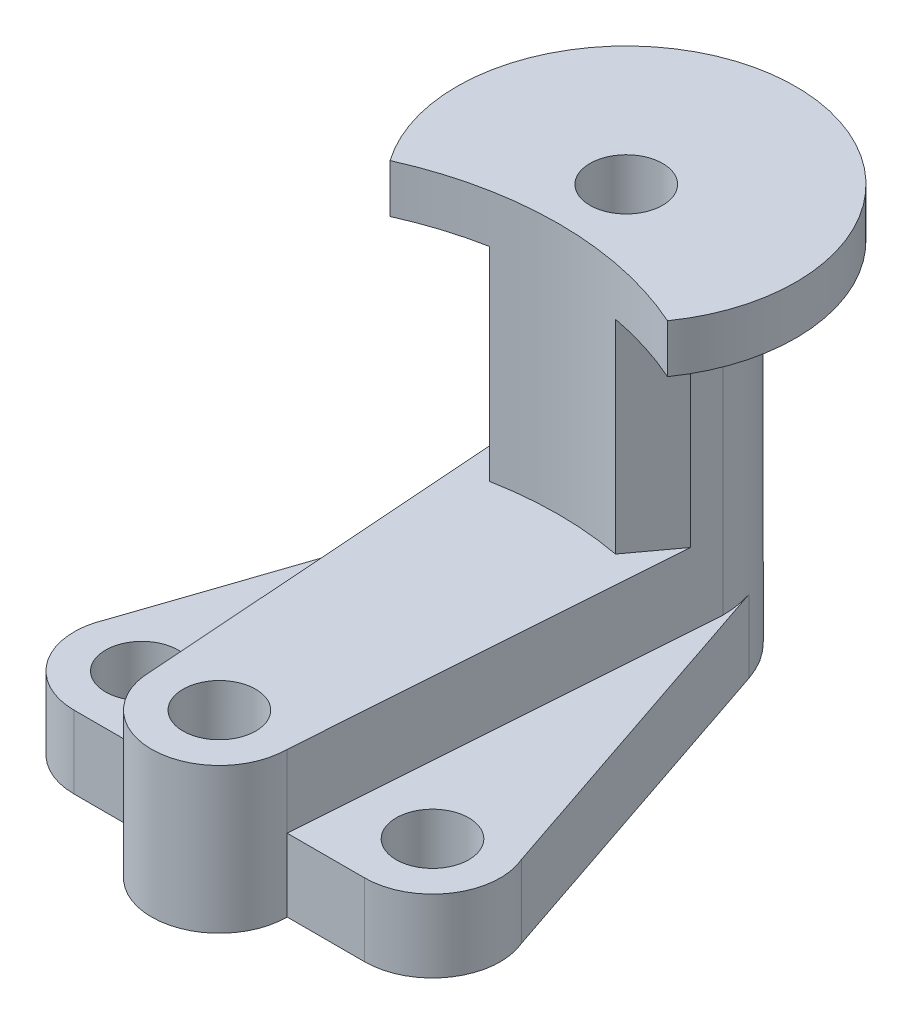
ISO-10303-21;
HEADER;
FILE_DESCRIPTION(('STEP AP214'),'2;1');
FILE_NAME('part.step','',(''),(''),'','','');
FILE_SCHEMA(('AUTOMOTIVE_DESIGN { 1 0 10303 214 1 1 1 1 }'));
ENDSEC;
DATA;
#1=APPLICATION_CONTEXT('core data for automotive mechanical design processes');
#2=APPLICATION_PROTOCOL_DEFINITION('international standard','automotive_design',2000,#1);
#3=PRODUCT_CONTEXT('',#1,'mechanical');
#4=PRODUCT('Part','Part','',(#3));
#5=PRODUCT_RELATED_PRODUCT_CATEGORY('part','',(#4));
#6=PRODUCT_DEFINITION_FORMATION('','',#4);
#7=PRODUCT_DEFINITION_CONTEXT('part definition',#1,'design');
#8=PRODUCT_DEFINITION('design','',#6,#7);
#9=PRODUCT_DEFINITION_SHAPE('','',#8);
#10=(LENGTH_UNIT() NAMED_UNIT(*) SI_UNIT(.MILLI.,.METRE.));
#11=(NAMED_UNIT(*) PLANE_ANGLE_UNIT() SI_UNIT($,.RADIAN.));
#12=(NAMED_UNIT(*) SI_UNIT($,.STERADIAN.) SOLID_ANGLE_UNIT());
#13=UNCERTAINTY_MEASURE_WITH_UNIT(LENGTH_MEASURE(1.E-05),#10,'distance_accuracy_value','');
#14=(GEOMETRIC_REPRESENTATION_CONTEXT(3) GLOBAL_UNCERTAINTY_ASSIGNED_CONTEXT((#13)) GLOBAL_UNIT_ASSIGNED_CONTEXT((#10,
#11,#12)) REPRESENTATION_CONTEXT('',''));
#15=CARTESIAN_POINT('',(0.,0.,0.));
#16=DIRECTION('',(0.,0.,1.));
#17=DIRECTION('',(1.,0.,0.));
#18=AXIS2_PLACEMENT_3D('',#15,#16,#17);
#19=CARTESIAN_POINT('',(0.,30.,0.));
#20=DIRECTION('',(0.,1.,0.));
#21=DIRECTION('',(0.,0.,1.));
#22=AXIS2_PLACEMENT_3D('',#19,#20,#21);
#23=PLANE('',#22);
#24=CARTESIAN_POINT('',(30.,30.,14.));
#25=DIRECTION('',(0.,1.,0.));
#26=DIRECTION('',(0.,0.,1.));
#27=AXIS2_PLACEMENT_3D('',#24,#25,#26);
#28=CIRCLE('',#27,7.50000000000001);
#29=CARTESIAN_POINT('',(30.,30.,21.5));
#30=VERTEX_POINT('',#29);
#31=EDGE_CURVE('E220',#30,#30,#28,.T.);
#32=ORIENTED_EDGE('',*,*,#31,.F.);
#33=EDGE_LOOP('',(#32));
#34=FACE_BOUND('',#33,.T.);
#35=CARTESIAN_POINT('',(30.,30.,14.));
#36=DIRECTION('',(0.,1.,0.));
#37=DIRECTION('',(0.,0.,1.));
#38=AXIS2_PLACEMENT_3D('',#35,#36,#37);
#39=CIRCLE('',#38,70.);
#40=CARTESIAN_POINT('',(42.9817375649056,30.,-54.7857142857143));
#41=VERTEX_POINT('',#40);
#42=CARTESIAN_POINT('',(17.0182624350943,30.,-54.7857142857143));
#43=VERTEX_POINT('',#42);
#44=EDGE_CURVE('E49',#41,#43,#39,.T.);
#45=ORIENTED_EDGE('',*,*,#44,.T.);
#46=DIRECTION('',(-0.592651717372166,0.,-0.805458839355446));
#47=VECTOR('',#46,1.);
#48=CARTESIAN_POINT('',(37.1931553721472,30.,-27.3664976144927));
#49=LINE('',#48,#47);
#50=CARTESIAN_POINT('',(10.4490124625655,30.,-63.7138255240829));
#51=VERTEX_POINT('',#50);
#52=EDGE_CURVE('E11',#43,#51,#49,.T.);
#53=ORIENTED_EDGE('',*,*,#52,.T.);
#54=DIRECTION('',(0.0712470499879096,0.,0.997458699830735));
#55=VECTOR('',#54,1.);
#56=CARTESIAN_POINT('',(14.9238578680203,30.,-1.06598984771573));
#57=LINE('',#56,#55);
#58=CARTESIAN_POINT('',(16.,30.,14.));
#59=VERTEX_POINT('',#58);
#60=EDGE_CURVE('E224',#51,#59,#57,.T.);
#61=ORIENTED_EDGE('',*,*,#60,.T.);
#62=CARTESIAN_POINT('',(30.,30.,14.));
#63=DIRECTION('',(0.,1.,0.));
#64=DIRECTION('',(0.,0.,1.));
#65=AXIS2_PLACEMENT_3D('',#62,#63,#64);
#66=CIRCLE('',#65,14.);
#67=CARTESIAN_POINT('',(44.,30.,14.));
#68=VERTEX_POINT('',#67);
#69=EDGE_CURVE('E223',#59,#68,#66,.T.);
#70=ORIENTED_EDGE('',*,*,#69,.T.);
#71=DIRECTION('',(0.0712470499879096,0.,-0.997458699830735));
#72=VECTOR('',#71,1.);
#73=CARTESIAN_POINT('',(44.7715736040609,30.,3.19796954314721));
#74=LINE('',#73,#72);
#75=CARTESIAN_POINT('',(49.5509875374345,30.,-63.7138255240829));
#76=VERTEX_POINT('',#75);
#77=EDGE_CURVE('E219',#68,#76,#74,.T.);
#78=ORIENTED_EDGE('',*,*,#77,.T.);
#79=DIRECTION('',(0.592651717372168,0.,-0.805458839355444));
#80=VECTOR('',#79,1.);
#81=CARTESIAN_POINT('',(1.7326811416019,30.,1.27489625050297));
#82=LINE('',#81,#80);
#83=EDGE_CURVE('E58',#41,#76,#82,.T.);
#84=ORIENTED_EDGE('',*,*,#83,.F.);
#85=EDGE_LOOP('',(#45,#53,#61,#70,#78,#84));
#86=FACE_BOUND('',#85,.T.);
#87=ADVANCED_FACE('F41',(#34,#86),#23,.T.);
#88=CARTESIAN_POINT('',(30.,15.,-70.));
#89=DIRECTION('',(0.,1.,0.));
#90=DIRECTION('',(0.,0.,1.));
#91=AXIS2_PLACEMENT_3D('',#88,#89,#90);
#92=PLANE('',#91);
#93=DIRECTION('',(1.,0.,0.));
#94=VECTOR('',#93,1.);
#95=CARTESIAN_POINT('',(0.,15.,14.));
#96=LINE('',#95,#94);
#97=CARTESIAN_POINT('',(22.5,15.,14.));
#98=VERTEX_POINT('',#97);
#99=CARTESIAN_POINT('',(37.5,15.,14.));
#100=VERTEX_POINT('',#99);
#101=EDGE_CURVE('E297',#98,#100,#96,.T.);
#102=ORIENTED_EDGE('',*,*,#101,.T.);
#103=CARTESIAN_POINT('',(30.,15.,14.));
#104=DIRECTION('',(0.,1.,0.));
#105=DIRECTION('',(0.,0.,1.));
#106=AXIS2_PLACEMENT_3D('',#103,#104,#105);
#107=CIRCLE('',#106,7.50000000000001);
#108=EDGE_CURVE('E207',#100,#98,#107,.T.);
#109=ORIENTED_EDGE('',*,*,#108,.T.);
#110=EDGE_LOOP('',(#102,#109));
#111=FACE_BOUND('',#110,.T.);
#112=ADVANCED_FACE('F385',(#111),#92,.T.);
#113=DIRECTION('',(0.0712470499879096,0.,-0.997458699830735));
#114=VECTOR('',#113,1.);
#115=CARTESIAN_POINT('',(44.7715736040609,15.,3.19796954314721));
#116=LINE('',#115,#114);
#117=CARTESIAN_POINT('',(44.,15.,14.));
#118=VERTEX_POINT('',#117);
#119=CARTESIAN_POINT('',(50.,15.,-70.));
#120=VERTEX_POINT('',#119);
#121=EDGE_CURVE('E229',#118,#120,#116,.T.);
#122=ORIENTED_EDGE('',*,*,#121,.F.);
#123=CARTESIAN_POINT('',(60.,15.,14.));
#124=VERTEX_POINT('',#123);
#125=EDGE_CURVE('E291',#118,#124,#96,.T.);
#126=ORIENTED_EDGE('',*,*,#125,.T.);
#127=CARTESIAN_POINT('',(60.,15.,0.));
#128=DIRECTION('',(0.,1.,0.));
#129=DIRECTION('',(0.,0.,1.));
#130=AXIS2_PLACEMENT_3D('',#127,#128,#129);
#131=CIRCLE('',#130,14.);
#132=CARTESIAN_POINT('',(72.8680304202528,15.,-5.51487018010835));
#133=VERTEX_POINT('',#132);
#134=EDGE_CURVE('E296',#124,#133,#131,.T.);
#135=ORIENTED_EDGE('',*,*,#134,.T.);
#136=DIRECTION('',(0.319730012709035,0.,0.947508690711109));
#137=VECTOR('',#136,1.);
#138=CARTESIAN_POINT('',(72.8680304202528,15.,-5.51487018010835));
#139=LINE('',#138,#137);
#140=CARTESIAN_POINT('',(48.9501738142222,15.,-76.3946002541807));
#141=VERTEX_POINT('',#140);
#142=EDGE_CURVE('E254',#141,#133,#139,.T.);
#143=ORIENTED_EDGE('',*,*,#142,.F.);
#144=CARTESIAN_POINT('',(30.,15.,-70.));
#145=DIRECTION('',(0.,1.,0.));
#146=DIRECTION('',(0.,0.,1.));
#147=AXIS2_PLACEMENT_3D('',#144,#145,#146);
#148=CIRCLE('',#147,20.);
#149=EDGE_CURVE('E233',#120,#141,#148,.T.);
#150=ORIENTED_EDGE('',*,*,#149,.F.);
#151=EDGE_LOOP('',(#122,#126,#135,#143,#150));
#152=FACE_BOUND('',#151,.T.);
#153=CARTESIAN_POINT('',(60.,15.,0.));
#154=DIRECTION('',(0.,1.,0.));
#155=DIRECTION('',(0.,0.,1.));
#156=AXIS2_PLACEMENT_3D('',#153,#154,#155);
#157=CIRCLE('',#156,7.5);
#158=CARTESIAN_POINT('',(60.,15.,7.5));
#159=VERTEX_POINT('',#158);
#160=EDGE_CURVE('E276',#159,#159,#157,.T.);
#161=ORIENTED_EDGE('',*,*,#160,.F.);
#162=EDGE_LOOP('',(#161));
#163=FACE_BOUND('',#162,.T.);
#164=ADVANCED_FACE('F388',(#152,#163),#92,.T.);
#165=CARTESIAN_POINT('',(0.,15.,14.));
#166=DIRECTION('',(0.,0.,-1.));
#167=DIRECTION('',(-1.,0.,0.));
#168=AXIS2_PLACEMENT_3D('',#165,#166,#167);
#169=PLANE('',#168);
#170=DIRECTION('',(0.,-1.,0.));
#171=VECTOR('',#170,1.);
#172=CARTESIAN_POINT('',(37.5,15.,14.));
#173=LINE('',#172,#171);
#174=CARTESIAN_POINT('',(37.5,0.,14.));
#175=VERTEX_POINT('',#174);
#176=EDGE_CURVE('E319',#100,#175,#173,.T.);
#177=ORIENTED_EDGE('',*,*,#176,.F.);
#178=ORIENTED_EDGE('',*,*,#101,.F.);
#179=DIRECTION('',(0.,-1.,0.));
#180=VECTOR('',#179,1.);
#181=CARTESIAN_POINT('',(22.5,15.,14.));
#182=LINE('',#181,#180);
#183=CARTESIAN_POINT('',(22.5,0.,14.));
#184=VERTEX_POINT('',#183);
#185=EDGE_CURVE('E318',#184,#98,#182,.F.);
#186=ORIENTED_EDGE('',*,*,#185,.F.);
#187=DIRECTION('',(1.,0.,0.));
#188=VECTOR('',#187,1.);
#189=CARTESIAN_POINT('',(0.,0.,14.));
#190=LINE('',#189,#188);
#191=EDGE_CURVE('E308',#184,#175,#190,.T.);
#192=ORIENTED_EDGE('',*,*,#191,.T.);
#193=EDGE_LOOP('',(#177,#178,#186,#192));
#194=FACE_BOUND('',#193,.T.);
#195=ADVANCED_FACE('F432',(#194),#169,.F.);
#196=ORIENTED_EDGE('',*,*,#125,.F.);
#197=DIRECTION('',(0.,-1.,0.));
#198=VECTOR('',#197,1.);
#199=CARTESIAN_POINT('',(44.,15.,14.));
#200=LINE('',#199,#198);
#201=CARTESIAN_POINT('',(44.,0.,14.));
#202=VERTEX_POINT('',#201);
#203=EDGE_CURVE('E273',#118,#202,#200,.T.);
#204=ORIENTED_EDGE('',*,*,#203,.T.);
#205=CARTESIAN_POINT('',(60.,0.,14.));
#206=VERTEX_POINT('',#205);
#207=EDGE_CURVE('E303',#202,#206,#190,.T.);
#208=ORIENTED_EDGE('',*,*,#207,.T.);
#209=DIRECTION('',(0.,-1.,0.));
#210=VECTOR('',#209,1.);
#211=CARTESIAN_POINT('',(60.,15.,14.));
#212=LINE('',#211,#210);
#213=EDGE_CURVE('E309',#124,#206,#212,.T.);
#214=ORIENTED_EDGE('',*,*,#213,.F.);
#215=EDGE_LOOP('',(#196,#204,#208,#214));
#216=FACE_BOUND('',#215,.T.);
#217=ADVANCED_FACE('F430',(#216),#169,.F.);
#218=DIRECTION('',(0.0712470499879096,0.,0.997458699830735));
#219=VECTOR('',#218,1.);
#220=CARTESIAN_POINT('',(14.9238578680203,15.,-1.06598984771573));
#221=LINE('',#220,#219);
#222=CARTESIAN_POINT('',(9.99999999999998,15.,-70.));
#223=VERTEX_POINT('',#222);
#224=CARTESIAN_POINT('',(16.,15.,14.));
#225=VERTEX_POINT('',#224);
#226=EDGE_CURVE('E222',#223,#225,#221,.T.);
#227=ORIENTED_EDGE('',*,*,#226,.F.);
#228=CARTESIAN_POINT('',(11.0498261857778,15.,-76.3946002541807));
#229=VERTEX_POINT('',#228);
#230=EDGE_CURVE('E237',#229,#223,#148,.T.);
#231=ORIENTED_EDGE('',*,*,#230,.F.);
#232=DIRECTION('',(0.319730012709035,0.,-0.947508690711109));
#233=VECTOR('',#232,1.);
#234=CARTESIAN_POINT('',(-12.8680304202528,15.,-5.51487018010835));
#235=LINE('',#234,#233);
#236=CARTESIAN_POINT('',(-12.8680304202528,15.,-5.51487018010835));
#237=VERTEX_POINT('',#236);
#238=EDGE_CURVE('E252',#237,#229,#235,.T.);
#239=ORIENTED_EDGE('',*,*,#238,.F.);
#240=CARTESIAN_POINT('',(0.,15.,0.));
#241=DIRECTION('',(0.,1.,0.));
#242=DIRECTION('',(0.,0.,1.));
#243=AXIS2_PLACEMENT_3D('',#240,#241,#242);
#244=CIRCLE('',#243,14.);
#245=CARTESIAN_POINT('',(0.,15.,14.));
#246=VERTEX_POINT('',#245);
#247=EDGE_CURVE('E292',#237,#246,#244,.T.);
#248=ORIENTED_EDGE('',*,*,#247,.T.);
#249=EDGE_CURVE('E293',#246,#225,#96,.T.);
#250=ORIENTED_EDGE('',*,*,#249,.T.);
#251=EDGE_LOOP('',(#227,#231,#239,#248,#250));
#252=FACE_BOUND('',#251,.T.);
#253=CARTESIAN_POINT('',(0.,15.,0.));
#254=DIRECTION('',(0.,1.,0.));
#255=DIRECTION('',(0.,0.,1.));
#256=AXIS2_PLACEMENT_3D('',#253,#254,#255);
#257=CIRCLE('',#256,7.5);
#258=CARTESIAN_POINT('',(0.,15.,7.5));
#259=VERTEX_POINT('',#258);
#260=EDGE_CURVE('E284',#259,#259,#257,.T.);
#261=ORIENTED_EDGE('',*,*,#260,.F.);
#262=EDGE_LOOP('',(#261));
#263=FACE_BOUND('',#262,.T.);
#264=ADVANCED_FACE('F340',(#252,#263),#92,.T.);
#265=CARTESIAN_POINT('',(30.,0.,-70.));
#266=DIRECTION('',(0.,1.,0.));
#267=DIRECTION('',(0.,0.,1.));
#268=AXIS2_PLACEMENT_3D('',#265,#266,#267);
#269=PLANE('',#268);
#270=CARTESIAN_POINT('',(30.,0.,-70.));
#271=DIRECTION('',(0.,1.,0.));
#272=DIRECTION('',(0.,0.,1.));
#273=AXIS2_PLACEMENT_3D('',#270,#271,#272);
#274=CIRCLE('',#273,7.5);
#275=CARTESIAN_POINT('',(30.,0.,-62.5));
#276=VERTEX_POINT('',#275);
#277=EDGE_CURVE('E44',#276,#276,#274,.T.);
#278=ORIENTED_EDGE('',*,*,#277,.T.);
#279=EDGE_LOOP('',(#278));
#280=FACE_BOUND('',#279,.T.);
#281=CARTESIAN_POINT('',(0.,0.,0.));
#282=DIRECTION('',(0.,1.,0.));
#283=DIRECTION('',(0.,0.,1.));
#284=AXIS2_PLACEMENT_3D('',#281,#282,#283);
#285=CIRCLE('',#284,14.);
#286=CARTESIAN_POINT('',(-12.8680304202528,0.,-5.51487018010835));
#287=VERTEX_POINT('',#286);
#288=CARTESIAN_POINT('',(0.,0.,14.));
#289=VERTEX_POINT('',#288);
#290=EDGE_CURVE('E288',#287,#289,#285,.T.);
#291=ORIENTED_EDGE('',*,*,#290,.F.);
#292=DIRECTION('',(0.319730012709035,0.,-0.947508690711109));
#293=VECTOR('',#292,1.);
#294=CARTESIAN_POINT('',(-12.8680304202528,0.,-5.51487018010835));
#295=LINE('',#294,#293);
#296=CARTESIAN_POINT('',(11.0498261857778,0.,-76.3946002541807));
#297=VERTEX_POINT('',#296);
#298=EDGE_CURVE('E253',#287,#297,#295,.T.);
#299=ORIENTED_EDGE('',*,*,#298,.T.);
#300=CARTESIAN_POINT('',(30.,0.,-70.));
#301=DIRECTION('',(0.,-1.,0.));
#302=DIRECTION('',(0.,0.,-1.));
#303=AXIS2_PLACEMENT_3D('',#300,#301,#302);
#304=CIRCLE('',#303,20.);
#305=CARTESIAN_POINT('',(48.9501738142222,0.,-76.3946002541807));
#306=VERTEX_POINT('',#305);
#307=EDGE_CURVE('E265',#297,#306,#304,.T.);
#308=ORIENTED_EDGE('',*,*,#307,.T.);
#309=DIRECTION('',(0.319730012709035,0.,0.947508690711109));
#310=VECTOR('',#309,1.);
#311=CARTESIAN_POINT('',(72.8680304202528,0.,-5.51487018010835));
#312=LINE('',#311,#310);
#313=CARTESIAN_POINT('',(72.8680304202528,0.,-5.51487018010835));
#314=VERTEX_POINT('',#313);
#315=EDGE_CURVE('E264',#306,#314,#312,.T.);
#316=ORIENTED_EDGE('',*,*,#315,.T.);
#317=CARTESIAN_POINT('',(60.,0.,0.));
#318=DIRECTION('',(0.,1.,0.));
#319=DIRECTION('',(0.,0.,1.));
#320=AXIS2_PLACEMENT_3D('',#317,#318,#319);
#321=CIRCLE('',#320,14.);
#322=EDGE_CURVE('E294',#206,#314,#321,.T.);
#323=ORIENTED_EDGE('',*,*,#322,.F.);
#324=ORIENTED_EDGE('',*,*,#207,.F.);
#325=CARTESIAN_POINT('',(30.,0.,14.));
#326=DIRECTION('',(0.,-1.,0.));
#327=DIRECTION('',(0.,0.,-1.));
#328=AXIS2_PLACEMENT_3D('',#325,#326,#327);
#329=CIRCLE('',#328,14.);
#330=CARTESIAN_POINT('',(16.,0.,14.));
#331=VERTEX_POINT('',#330);
#332=EDGE_CURVE('E258',#202,#331,#329,.T.);
#333=ORIENTED_EDGE('',*,*,#332,.T.);
#334=EDGE_CURVE('E304',#289,#331,#190,.T.);
#335=ORIENTED_EDGE('',*,*,#334,.F.);
#336=EDGE_LOOP('',(#291,#299,#308,#316,#323,#324,#333,#335));
#337=FACE_BOUND('',#336,.T.);
#338=CARTESIAN_POINT('',(30.,0.,14.));
#339=DIRECTION('',(0.,-1.,0.));
#340=DIRECTION('',(0.,0.,-1.));
#341=AXIS2_PLACEMENT_3D('',#338,#339,#340);
#342=CIRCLE('',#341,7.5);
#343=EDGE_CURVE('E248',#175,#184,#342,.T.);
#344=ORIENTED_EDGE('',*,*,#343,.F.);
#345=ORIENTED_EDGE('',*,*,#191,.F.);
#346=EDGE_LOOP('',(#344,#345));
#347=FACE_BOUND('',#346,.T.);
#348=CARTESIAN_POINT('',(0.,0.,0.));
#349=DIRECTION('',(0.,1.,0.));
#350=DIRECTION('',(0.,0.,1.));
#351=AXIS2_PLACEMENT_3D('',#348,#349,#350);
#352=CIRCLE('',#351,7.5);
#353=CARTESIAN_POINT('',(0.,0.,7.5));
#354=VERTEX_POINT('',#353);
#355=EDGE_CURVE('E285',#354,#354,#352,.T.);
#356=ORIENTED_EDGE('',*,*,#355,.T.);
#357=EDGE_LOOP('',(#356));
#358=FACE_BOUND('',#357,.T.);
#359=CARTESIAN_POINT('',(60.,0.,0.));
#360=DIRECTION('',(0.,1.,0.));
#361=DIRECTION('',(0.,0.,1.));
#362=AXIS2_PLACEMENT_3D('',#359,#360,#361);
#363=CIRCLE('',#362,7.5);
#364=CARTESIAN_POINT('',(60.,0.,7.5));
#365=VERTEX_POINT('',#364);
#366=EDGE_CURVE('E272',#365,#365,#363,.T.);
#367=ORIENTED_EDGE('',*,*,#366,.T.);
#368=EDGE_LOOP('',(#367));
#369=FACE_BOUND('',#368,.T.);
#370=ADVANCED_FACE('F369',(#280,#337,#347,#358,#369),#269,.F.);
#371=CARTESIAN_POINT('',(0.,15.,0.));
#372=DIRECTION('',(0.,-1.,0.));
#373=DIRECTION('',(0.,0.,-1.));
#374=AXIS2_PLACEMENT_3D('',#371,#372,#373);
#375=CYLINDRICAL_SURFACE('',#374,14.);
#376=ORIENTED_EDGE('',*,*,#290,.T.);
#377=DIRECTION('',(0.,-1.,0.));
#378=VECTOR('',#377,1.);
#379=CARTESIAN_POINT('',(0.,15.,14.));
#380=LINE('',#379,#378);
#381=EDGE_CURVE('E311',#246,#289,#380,.T.);
#382=ORIENTED_EDGE('',*,*,#381,.F.);
#383=ORIENTED_EDGE('',*,*,#247,.F.);
#384=DIRECTION('',(0.,-1.,0.));
#385=VECTOR('',#384,1.);
#386=CARTESIAN_POINT('',(-12.8680304202528,15.,-5.51487018010835));
#387=LINE('',#386,#385);
#388=EDGE_CURVE('E316',#237,#287,#387,.T.);
#389=ORIENTED_EDGE('',*,*,#388,.T.);
#390=EDGE_LOOP('',(#376,#382,#383,#389));
#391=FACE_BOUND('',#390,.T.);
#392=ADVANCED_FACE('F43',(#391),#375,.T.);
#393=ORIENTED_EDGE('',*,*,#334,.T.);
#394=DIRECTION('',(0.,-1.,0.));
#395=VECTOR('',#394,1.);
#396=CARTESIAN_POINT('',(16.,15.,14.));
#397=LINE('',#396,#395);
#398=EDGE_CURVE('E269',#225,#331,#397,.T.);
#399=ORIENTED_EDGE('',*,*,#398,.F.);
#400=ORIENTED_EDGE('',*,*,#249,.F.);
#401=ORIENTED_EDGE('',*,*,#381,.T.);
#402=EDGE_LOOP('',(#393,#399,#400,#401));
#403=FACE_BOUND('',#402,.T.);
#404=ADVANCED_FACE('F429',(#403),#169,.F.);
#405=CARTESIAN_POINT('',(60.,15.,0.));
#406=DIRECTION('',(0.,-1.,0.));
#407=DIRECTION('',(0.,0.,-1.));
#408=AXIS2_PLACEMENT_3D('',#405,#406,#407);
#409=CYLINDRICAL_SURFACE('',#408,14.);
#410=ORIENTED_EDGE('',*,*,#322,.T.);
#411=DIRECTION('',(0.,-1.,0.));
#412=VECTOR('',#411,1.);
#413=CARTESIAN_POINT('',(72.8680304202528,15.,-5.51487018010835));
#414=LINE('',#413,#412);
#415=EDGE_CURVE('E302',#133,#314,#414,.T.);
#416=ORIENTED_EDGE('',*,*,#415,.F.);
#417=ORIENTED_EDGE('',*,*,#134,.F.);
#418=ORIENTED_EDGE('',*,*,#213,.T.);
#419=EDGE_LOOP('',(#410,#416,#417,#418));
#420=FACE_BOUND('',#419,.T.);
#421=ADVANCED_FACE('F421',(#420),#409,.T.);
#422=CARTESIAN_POINT('',(0.,15.,0.));
#423=DIRECTION('',(0.,-1.,0.));
#424=DIRECTION('',(0.,0.,-1.));
#425=AXIS2_PLACEMENT_3D('',#422,#423,#424);
#426=CYLINDRICAL_SURFACE('',#425,7.5);
#427=ORIENTED_EDGE('',*,*,#260,.T.);
#428=EDGE_LOOP('',(#427));
#429=FACE_BOUND('',#428,.T.);
#430=ORIENTED_EDGE('',*,*,#355,.F.);
#431=EDGE_LOOP('',(#430));
#432=FACE_BOUND('',#431,.T.);
#433=ADVANCED_FACE('F419',(#429,#432),#426,.F.);
#434=CARTESIAN_POINT('',(60.,15.,0.));
#435=DIRECTION('',(0.,-1.,0.));
#436=DIRECTION('',(0.,0.,-1.));
#437=AXIS2_PLACEMENT_3D('',#434,#435,#436);
#438=CYLINDRICAL_SURFACE('',#437,7.5);
#439=ORIENTED_EDGE('',*,*,#160,.T.);
#440=EDGE_LOOP('',(#439));
#441=FACE_BOUND('',#440,.T.);
#442=ORIENTED_EDGE('',*,*,#366,.F.);
#443=EDGE_LOOP('',(#442));
#444=FACE_BOUND('',#443,.T.);
#445=ADVANCED_FACE('F418',(#441,#444),#438,.F.);
#446=CARTESIAN_POINT('',(-12.8680304202528,15.,-5.51487018010835));
#447=DIRECTION('',(-0.947508690711109,0.,-0.319730012709035));
#448=DIRECTION('',(-0.319730012709035,0.,0.947508690711109));
#449=AXIS2_PLACEMENT_3D('',#446,#447,#448);
#450=PLANE('',#449);
#451=ORIENTED_EDGE('',*,*,#298,.F.);
#452=ORIENTED_EDGE('',*,*,#388,.F.);
#453=ORIENTED_EDGE('',*,*,#238,.T.);
#454=DIRECTION('',(0.,-1.,0.));
#455=VECTOR('',#454,1.);
#456=CARTESIAN_POINT('',(11.0498261857778,15.,-76.3946002541807));
#457=LINE('',#456,#455);
#458=EDGE_CURVE('E259',#229,#297,#457,.T.);
#459=ORIENTED_EDGE('',*,*,#458,.T.);
#460=EDGE_LOOP('',(#451,#452,#453,#459));
#461=FACE_BOUND('',#460,.T.);
#462=ADVANCED_FACE('F413',(#461),#450,.T.);
#463=CARTESIAN_POINT('',(30.,15.,-70.));
#464=DIRECTION('',(0.,-1.,0.));
#465=DIRECTION('',(0.,0.,-1.));
#466=AXIS2_PLACEMENT_3D('',#463,#464,#465);
#467=CYLINDRICAL_SURFACE('',#466,20.);
#468=DIRECTION('',(0.,-1.,0.));
#469=VECTOR('',#468,1.);
#470=CARTESIAN_POINT('',(50.,30.,-70.));
#471=LINE('',#470,#469);
#472=CARTESIAN_POINT('',(50.,72.,-70.));
#473=VERTEX_POINT('',#472);
#474=EDGE_CURVE('E247',#473,#120,#471,.T.);
#475=ORIENTED_EDGE('',*,*,#474,.T.);
#476=ORIENTED_EDGE('',*,*,#149,.T.);
#477=DIRECTION('',(0.,-1.,0.));
#478=VECTOR('',#477,1.);
#479=CARTESIAN_POINT('',(48.9501738142222,15.,-76.3946002541807));
#480=LINE('',#479,#478);
#481=EDGE_CURVE('E277',#141,#306,#480,.T.);
#482=ORIENTED_EDGE('',*,*,#481,.T.);
#483=ORIENTED_EDGE('',*,*,#307,.F.);
#484=ORIENTED_EDGE('',*,*,#458,.F.);
#485=ORIENTED_EDGE('',*,*,#230,.T.);
#486=DIRECTION('',(0.,-1.,0.));
#487=VECTOR('',#486,1.);
#488=CARTESIAN_POINT('',(9.99999999999998,30.,-70.));
#489=LINE('',#488,#487);
#490=CARTESIAN_POINT('',(9.99999999999998,72.,-70.));
#491=VERTEX_POINT('',#490);
#492=EDGE_CURVE('E242',#491,#223,#489,.T.);
#493=ORIENTED_EDGE('',*,*,#492,.F.);
#494=CARTESIAN_POINT('',(30.,72.,-70.));
#495=DIRECTION('',(0.,1.,0.));
#496=DIRECTION('',(0.,0.,1.));
#497=AXIS2_PLACEMENT_3D('',#494,#495,#496);
#498=CIRCLE('',#497,20.);
#499=EDGE_CURVE('E197',#473,#491,#498,.T.);
#500=ORIENTED_EDGE('',*,*,#499,.F.);
#501=EDGE_LOOP('',(#475,#476,#482,#483,#484,#485,#493,#500));
#502=FACE_BOUND('',#501,.T.);
#503=ADVANCED_FACE('F332',(#502),#467,.T.);
#504=CARTESIAN_POINT('',(72.8680304202528,15.,-5.51487018010835));
#505=DIRECTION('',(0.947508690711109,0.,-0.319730012709035));
#506=DIRECTION('',(-0.319730012709035,0.,-0.947508690711109));
#507=AXIS2_PLACEMENT_3D('',#504,#505,#506);
#508=PLANE('',#507);
#509=ORIENTED_EDGE('',*,*,#315,.F.);
#510=ORIENTED_EDGE('',*,*,#481,.F.);
#511=ORIENTED_EDGE('',*,*,#142,.T.);
#512=ORIENTED_EDGE('',*,*,#415,.T.);
#513=EDGE_LOOP('',(#509,#510,#511,#512));
#514=FACE_BOUND('',#513,.T.);
#515=ADVANCED_FACE('F408',(#514),#508,.T.);
#516=CARTESIAN_POINT('',(30.,15.,14.));
#517=DIRECTION('',(0.,-1.,0.));
#518=DIRECTION('',(0.,0.,-1.));
#519=AXIS2_PLACEMENT_3D('',#516,#517,#518);
#520=CYLINDRICAL_SURFACE('',#519,7.5);
#521=ORIENTED_EDGE('',*,*,#185,.T.);
#522=ORIENTED_EDGE('',*,*,#108,.F.);
#523=ORIENTED_EDGE('',*,*,#176,.T.);
#524=ORIENTED_EDGE('',*,*,#343,.T.);
#525=EDGE_LOOP('',(#521,#522,#523,#524));
#526=FACE_BOUND('',#525,.T.);
#527=ORIENTED_EDGE('',*,*,#31,.T.);
#528=EDGE_LOOP('',(#527));
#529=FACE_BOUND('',#528,.T.);
#530=ADVANCED_FACE('F401',(#526,#529),#520,.F.);
#531=CARTESIAN_POINT('',(30.,15.,14.));
#532=DIRECTION('',(0.,-1.,0.));
#533=DIRECTION('',(0.,0.,-1.));
#534=AXIS2_PLACEMENT_3D('',#531,#532,#533);
#535=CYLINDRICAL_SURFACE('',#534,14.);
#536=ORIENTED_EDGE('',*,*,#332,.F.);
#537=ORIENTED_EDGE('',*,*,#203,.F.);
#538=DIRECTION('',(0.,-1.,0.));
#539=VECTOR('',#538,1.);
#540=CARTESIAN_POINT('',(44.,30.,14.));
#541=LINE('',#540,#539);
#542=EDGE_CURVE('E230',#68,#118,#541,.T.);
#543=ORIENTED_EDGE('',*,*,#542,.F.);
#544=ORIENTED_EDGE('',*,*,#69,.F.);
#545=DIRECTION('',(0.,-1.,0.));
#546=VECTOR('',#545,1.);
#547=CARTESIAN_POINT('',(16.,30.,14.));
#548=LINE('',#547,#546);
#549=EDGE_CURVE('E243',#59,#225,#548,.T.);
#550=ORIENTED_EDGE('',*,*,#549,.T.);
#551=ORIENTED_EDGE('',*,*,#398,.T.);
#552=EDGE_LOOP('',(#536,#537,#543,#544,#550,#551));
#553=FACE_BOUND('',#552,.T.);
#554=ADVANCED_FACE('F350',(#553),#535,.T.);
#555=CARTESIAN_POINT('',(44.7715736040609,30.,3.19796954314721));
#556=DIRECTION('',(-0.997458699830735,0.,-0.0712470499879096));
#557=DIRECTION('',(-0.0712470499879096,0.,0.997458699830735));
#558=AXIS2_PLACEMENT_3D('',#555,#556,#557);
#559=PLANE('',#558);
#560=DIRECTION('',(0.,1.,0.));
#561=VECTOR('',#560,1.);
#562=CARTESIAN_POINT('',(49.5509875374345,22.,-63.7138255240829));
#563=LINE('',#562,#561);
#564=CARTESIAN_POINT('',(49.5509875374345,72.,-63.7138255240829));
#565=VERTEX_POINT('',#564);
#566=EDGE_CURVE('E213',#76,#565,#563,.T.);
#567=ORIENTED_EDGE('',*,*,#566,.F.);
#568=ORIENTED_EDGE('',*,*,#77,.F.);
#569=ORIENTED_EDGE('',*,*,#542,.T.);
#570=ORIENTED_EDGE('',*,*,#121,.T.);
#571=ORIENTED_EDGE('',*,*,#474,.F.);
#572=DIRECTION('',(0.0712470499879103,0.,-0.997458699830735));
#573=VECTOR('',#572,1.);
#574=CARTESIAN_POINT('',(44.7715736040609,72.,3.19796954314723));
#575=LINE('',#574,#573);
#576=EDGE_CURVE('E192',#565,#473,#575,.T.);
#577=ORIENTED_EDGE('',*,*,#576,.F.);
#578=EDGE_LOOP('',(#567,#568,#569,#570,#571,#577));
#579=FACE_BOUND('',#578,.T.);
#580=ADVANCED_FACE('F399',(#579),#559,.F.);
#581=CARTESIAN_POINT('',(14.9238578680203,30.,-1.06598984771573));
#582=DIRECTION('',(0.997458699830735,0.,-0.0712470499879096));
#583=DIRECTION('',(-0.0712470499879096,0.,-0.997458699830735));
#584=AXIS2_PLACEMENT_3D('',#581,#582,#583);
#585=PLANE('',#584);
#586=ORIENTED_EDGE('',*,*,#60,.F.);
#587=DIRECTION('',(0.,1.,0.));
#588=VECTOR('',#587,1.);
#589=CARTESIAN_POINT('',(10.4490124625655,22.,-63.7138255240829));
#590=LINE('',#589,#588);
#591=CARTESIAN_POINT('',(10.4490124625655,72.,-63.7138255240829));
#592=VERTEX_POINT('',#591);
#593=EDGE_CURVE('E209',#51,#592,#590,.T.);
#594=ORIENTED_EDGE('',*,*,#593,.T.);
#595=DIRECTION('',(-0.0712470499879097,0.,-0.997458699830735));
#596=VECTOR('',#595,1.);
#597=CARTESIAN_POINT('',(14.9238578680203,72.,-1.06598984771574));
#598=LINE('',#597,#596);
#599=EDGE_CURVE('E200',#592,#491,#598,.T.);
#600=ORIENTED_EDGE('',*,*,#599,.T.);
#601=ORIENTED_EDGE('',*,*,#492,.T.);
#602=ORIENTED_EDGE('',*,*,#226,.T.);
#603=ORIENTED_EDGE('',*,*,#549,.F.);
#604=EDGE_LOOP('',(#586,#594,#600,#601,#602,#603));
#605=FACE_BOUND('',#604,.T.);
#606=ADVANCED_FACE('F343',(#605),#585,.F.);
#607=CARTESIAN_POINT('',(30.,22.,14.));
#608=DIRECTION('',(0.,1.,0.));
#609=DIRECTION('',(0.,0.,1.));
#610=AXIS2_PLACEMENT_3D('',#607,#608,#609);
#611=CYLINDRICAL_SURFACE('',#610,70.);
#612=ORIENTED_EDGE('',*,*,#44,.F.);
#613=DIRECTION('',(0.,1.,0.));
#614=VECTOR('',#613,1.);
#615=CARTESIAN_POINT('',(42.9817375649056,22.,-54.7857142857143));
#616=LINE('',#615,#614);
#617=CARTESIAN_POINT('',(42.9817375649056,72.,-54.7857142857143));
#618=VERTEX_POINT('',#617);
#619=EDGE_CURVE('E202',#41,#618,#616,.T.);
#620=ORIENTED_EDGE('',*,*,#619,.T.);
#621=CARTESIAN_POINT('',(30.,72.,14.));
#622=DIRECTION('',(0.,-1.,0.));
#623=DIRECTION('',(0.,0.,1.));
#624=AXIS2_PLACEMENT_3D('',#621,#622,#623);
#625=CIRCLE('',#624,70.);
#626=CARTESIAN_POINT('',(58.6353693009188,72.,-49.875));
#627=VERTEX_POINT('',#626);
#628=EDGE_CURVE('E190',#618,#627,#625,.T.);
#629=ORIENTED_EDGE('',*,*,#628,.T.);
#630=DIRECTION('',(0.,-1.,0.));
#631=VECTOR('',#630,1.);
#632=CARTESIAN_POINT('',(58.6353693009188,82.,-49.875));
#633=LINE('',#632,#631);
#634=CARTESIAN_POINT('',(58.6353693009188,82.,-49.875));
#635=VERTEX_POINT('',#634);
#636=EDGE_CURVE('E171',#635,#627,#633,.T.);
#637=ORIENTED_EDGE('',*,*,#636,.F.);
#638=CARTESIAN_POINT('',(30.,82.,14.));
#639=DIRECTION('',(0.,-1.,0.));
#640=DIRECTION('',(0.,0.,1.));
#641=AXIS2_PLACEMENT_3D('',#638,#639,#640);
#642=CIRCLE('',#641,70.);
#643=CARTESIAN_POINT('',(1.3646306990812,82.,-49.875));
#644=VERTEX_POINT('',#643);
#645=EDGE_CURVE('E178',#644,#635,#642,.T.);
#646=ORIENTED_EDGE('',*,*,#645,.F.);
#647=DIRECTION('',(0.,-1.,0.));
#648=VECTOR('',#647,1.);
#649=CARTESIAN_POINT('',(1.3646306990812,82.,-49.875));
#650=LINE('',#649,#648);
#651=CARTESIAN_POINT('',(1.3646306990812,72.,-49.875));
#652=VERTEX_POINT('',#651);
#653=EDGE_CURVE('E174',#644,#652,#650,.T.);
#654=ORIENTED_EDGE('',*,*,#653,.T.);
#655=CARTESIAN_POINT('',(17.0182624350943,72.,-54.7857142857143));
#656=VERTEX_POINT('',#655);
#657=EDGE_CURVE('E359',#652,#656,#625,.T.);
#658=ORIENTED_EDGE('',*,*,#657,.T.);
#659=DIRECTION('',(0.,1.,0.));
#660=VECTOR('',#659,1.);
#661=CARTESIAN_POINT('',(17.0182624350943,22.,-54.7857142857143));
#662=LINE('',#661,#660);
#663=EDGE_CURVE('E206',#43,#656,#662,.T.);
#664=ORIENTED_EDGE('',*,*,#663,.F.);
#665=EDGE_LOOP('',(#612,#620,#629,#637,#646,#654,#658,#664));
#666=FACE_BOUND('',#665,.T.);
#667=ADVANCED_FACE('F183',(#666),#611,.F.);
#668=CARTESIAN_POINT('',(37.1931553721472,22.,-27.3664976144927));
#669=DIRECTION('',(0.805458839355446,0.,-0.592651717372166));
#670=DIRECTION('',(-0.592651717372166,0.,-0.805458839355446));
#671=AXIS2_PLACEMENT_3D('',#668,#669,#670);
#672=PLANE('',#671);
#673=ORIENTED_EDGE('',*,*,#52,.F.);
#674=ORIENTED_EDGE('',*,*,#663,.T.);
#675=DIRECTION('',(-0.592651717372166,0.,-0.805458839355446));
#676=VECTOR('',#675,1.);
#677=CARTESIAN_POINT('',(37.1931553721472,72.,-27.3664976144927));
#678=LINE('',#677,#676);
#679=EDGE_CURVE('E205',#656,#592,#678,.T.);
#680=ORIENTED_EDGE('',*,*,#679,.T.);
#681=ORIENTED_EDGE('',*,*,#593,.F.);
#682=EDGE_LOOP('',(#673,#674,#680,#681));
#683=FACE_BOUND('',#682,.T.);
#684=ADVANCED_FACE('F351',(#683),#672,.F.);
#685=CARTESIAN_POINT('',(1.7326811416019,22.,1.27489625050297));
#686=DIRECTION('',(0.805458839355444,0.,0.592651717372168));
#687=DIRECTION('',(0.592651717372168,0.,-0.805458839355444));
#688=AXIS2_PLACEMENT_3D('',#685,#686,#687);
#689=PLANE('',#688);
#690=ORIENTED_EDGE('',*,*,#619,.F.);
#691=ORIENTED_EDGE('',*,*,#83,.T.);
#692=ORIENTED_EDGE('',*,*,#566,.T.);
#693=DIRECTION('',(0.592651717372168,0.,-0.805458839355444));
#694=VECTOR('',#693,1.);
#695=CARTESIAN_POINT('',(1.7326811416019,72.,1.27489625050297));
#696=LINE('',#695,#694);
#697=EDGE_CURVE('E187',#618,#565,#696,.T.);
#698=ORIENTED_EDGE('',*,*,#697,.F.);
#699=EDGE_LOOP('',(#690,#691,#692,#698));
#700=FACE_BOUND('',#699,.T.);
#701=ADVANCED_FACE('F453',(#700),#689,.T.);
#702=CARTESIAN_POINT('',(30.,72.,-28.));
#703=DIRECTION('',(0.,1.,0.));
#704=DIRECTION('',(0.,0.,1.));
#705=AXIS2_PLACEMENT_3D('',#702,#703,#704);
#706=PLANE('',#705);
#707=ORIENTED_EDGE('',*,*,#628,.F.);
#708=ORIENTED_EDGE('',*,*,#697,.T.);
#709=ORIENTED_EDGE('',*,*,#576,.T.);
#710=ORIENTED_EDGE('',*,*,#499,.T.);
#711=ORIENTED_EDGE('',*,*,#599,.F.);
#712=ORIENTED_EDGE('',*,*,#679,.F.);
#713=ORIENTED_EDGE('',*,*,#657,.F.);
#714=CARTESIAN_POINT('',(30.,72.,-70.));
#715=DIRECTION('',(0.,1.,0.));
#716=DIRECTION('',(0.,0.,1.));
#717=AXIS2_PLACEMENT_3D('',#714,#715,#716);
#718=CIRCLE('',#717,35.);
#719=EDGE_CURVE('E181',#627,#652,#718,.T.);
#720=ORIENTED_EDGE('',*,*,#719,.F.);
#721=EDGE_LOOP('',(#707,#708,#709,#710,#711,#712,#713,#720));
#722=FACE_BOUND('',#721,.T.);
#723=ADVANCED_FACE('F358',(#722),#706,.F.);
#724=CARTESIAN_POINT('',(30.,82.,-28.));
#725=DIRECTION('',(0.,1.,0.));
#726=DIRECTION('',(0.,0.,1.));
#727=AXIS2_PLACEMENT_3D('',#724,#725,#726);
#728=PLANE('',#727);
#729=ORIENTED_EDGE('',*,*,#645,.T.);
#730=CARTESIAN_POINT('',(30.,82.,-70.));
#731=DIRECTION('',(0.,1.,0.));
#732=DIRECTION('',(0.,0.,1.));
#733=AXIS2_PLACEMENT_3D('',#730,#731,#732);
#734=CIRCLE('',#733,35.);
#735=EDGE_CURVE('E166',#635,#644,#734,.T.);
#736=ORIENTED_EDGE('',*,*,#735,.T.);
#737=EDGE_LOOP('',(#729,#736));
#738=FACE_BOUND('',#737,.T.);
#739=CARTESIAN_POINT('',(30.,82.,-70.));
#740=DIRECTION('',(0.,1.,0.));
#741=DIRECTION('',(0.,0.,1.));
#742=AXIS2_PLACEMENT_3D('',#739,#740,#741);
#743=CIRCLE('',#742,7.49999999999999);
#744=CARTESIAN_POINT('',(30.,82.,-62.5));
#745=VERTEX_POINT('',#744);
#746=EDGE_CURVE('E363',#745,#745,#743,.T.);
#747=ORIENTED_EDGE('',*,*,#746,.F.);
#748=EDGE_LOOP('',(#747));
#749=FACE_BOUND('',#748,.T.);
#750=ADVANCED_FACE('F176',(#738,#749),#728,.T.);
#751=CARTESIAN_POINT('',(30.,82.,-70.));
#752=DIRECTION('',(0.,-1.,0.));
#753=DIRECTION('',(0.,0.,-1.));
#754=AXIS2_PLACEMENT_3D('',#751,#752,#753);
#755=CYLINDRICAL_SURFACE('',#754,35.);
#756=ORIENTED_EDGE('',*,*,#719,.T.);
#757=ORIENTED_EDGE('',*,*,#653,.F.);
#758=ORIENTED_EDGE('',*,*,#735,.F.);
#759=ORIENTED_EDGE('',*,*,#636,.T.);
#760=EDGE_LOOP('',(#756,#757,#758,#759));
#761=FACE_BOUND('',#760,.T.);
#762=ADVANCED_FACE('F173',(#761),#755,.T.);
#763=CARTESIAN_POINT('',(30.,22.,-70.));
#764=DIRECTION('',(0.,1.,0.));
#765=DIRECTION('',(0.,0.,1.));
#766=AXIS2_PLACEMENT_3D('',#763,#764,#765);
#767=CYLINDRICAL_SURFACE('',#766,7.5);
#768=ORIENTED_EDGE('',*,*,#746,.T.);
#769=EDGE_LOOP('',(#768));
#770=FACE_BOUND('',#769,.T.);
#771=ORIENTED_EDGE('',*,*,#277,.F.);
#772=EDGE_LOOP('',(#771));
#773=FACE_BOUND('',#772,.T.);
#774=ADVANCED_FACE('F375',(#770,#773),#767,.F.);
#775=CLOSED_SHELL('',(#87,#112,#164,#195,#217,#264,#370,#392,#404,#421,#433,#445,#462,#503,#515,
#530,#554,#580,#606,#667,#684,#701,#723,#750,#762,#774));
#776=MANIFOLD_SOLID_BREP('B2',#775);
#777=ADVANCED_BREP_SHAPE_REPRESENTATION('',(#18,#776),#14);
#778=SHAPE_DEFINITION_REPRESENTATION(#9,#777);
ENDSEC;
END-ISO-10303-21;
